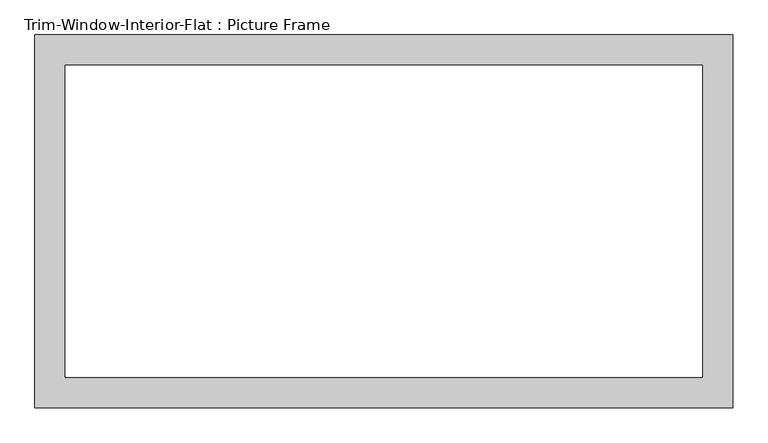
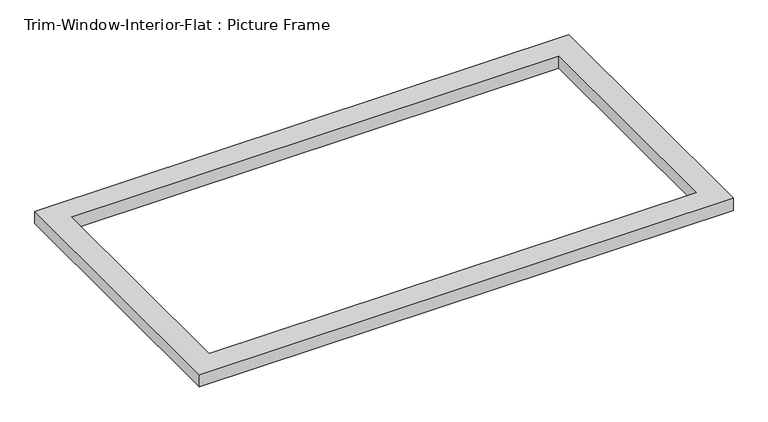
"""IFC4 building model written with IfcOpenShell, lengths in millimetres: proxy geometry, Trim-Window-Interior-Flat : Picture Frame."""

from ifc_helpers import new_model, si_unit, origin, origin_with_axes, place, context, project, spatial, polyline, outline, extrude, source, transform, mapped, element, save


def trim_window_interior_flat_picture_frame_0870d947(model_context):
    return source(origin(), model_context, "Body", "SweptSolid", [
        extrude(outline(polyline([(654.05, 44.45), (654.05, -654.05), (-654.05, -654.05), (-654.05, 44.45), (654.05, 44.45)]), holes=[polyline([(596.9, -12.7), (-596.9, -12.7), (-596.9, -596.9), (596.9, -596.9), (596.9, -12.7)])]), origin_with_axes(), (0.0, 0.0, 1.0), 31.75),
    ])


if __name__ == "__main__":
    model = new_model("IFC4")
    model_context = context("Model", 3, world=origin())
    ifc_project = project(units=[si_unit("LENGTHUNIT", "METRE", prefix="MILLI")], contexts=[model_context])
    site = spatial("IfcSite", under=ifc_project)
    building = spatial("IfcBuilding", under=site)
    placement = place(None, origin())
    trim_window_interior_flat_picture_frame_shape = trim_window_interior_flat_picture_frame_0870d947(model_context)
    element("IfcBuildingElementProxy", 1, Name="Trim-Window-Interior-Flat : Picture Frame", ObjectType="Trim-Window-Interior-Flat : Picture Frame", at=placement, inside=building, context=model_context, shape_type="MappedRepresentation", body=[
        mapped(trim_window_interior_flat_picture_frame_shape, transform((0.0, 0.0, 0.0), x_axis=(1.0, 0.0, 0.0), y_axis=(0.0, 1.0, 0.0), z_axis=(0.0, 0.0, 1.0))),
    ])
    save(model, "model.ifc")

# Revit data of these elements
# Type "Trim-Window-Interior-Flat : Picture Frame"
#   Trim Thickness_Picture Frame = 0' - 1 1/4"
#   Trim Width = 0' - 2 1/4"
#   Trim Thickness_with Sill = 0' - 0 3/4"
#   Sill Thickness = 0' - 1 1/4"
#   Opening Width [instance default] = 2' - 0"
#   Opening Height [instance default] = 3' - 0"
#   Default Elevation = 4' - 0"
#   Sill = no
#   Picture Frame = yes
#   Trim Material [instance default] = none
# Element 1 (IfcBuildingElementProxy, "Trim-Window-Interior-Flat : Picture Frame")
#   Opening Width = 4' - 0"
#   Opening Height = 2' - 0"
#   Trim Material = Wood - Stained
#   Materials on its faces: "Wood - Stained"
# Materials
#   "Wood - Stained": class "Wood", colour RGB 224 178 126, transparency 0, Cost = 0
